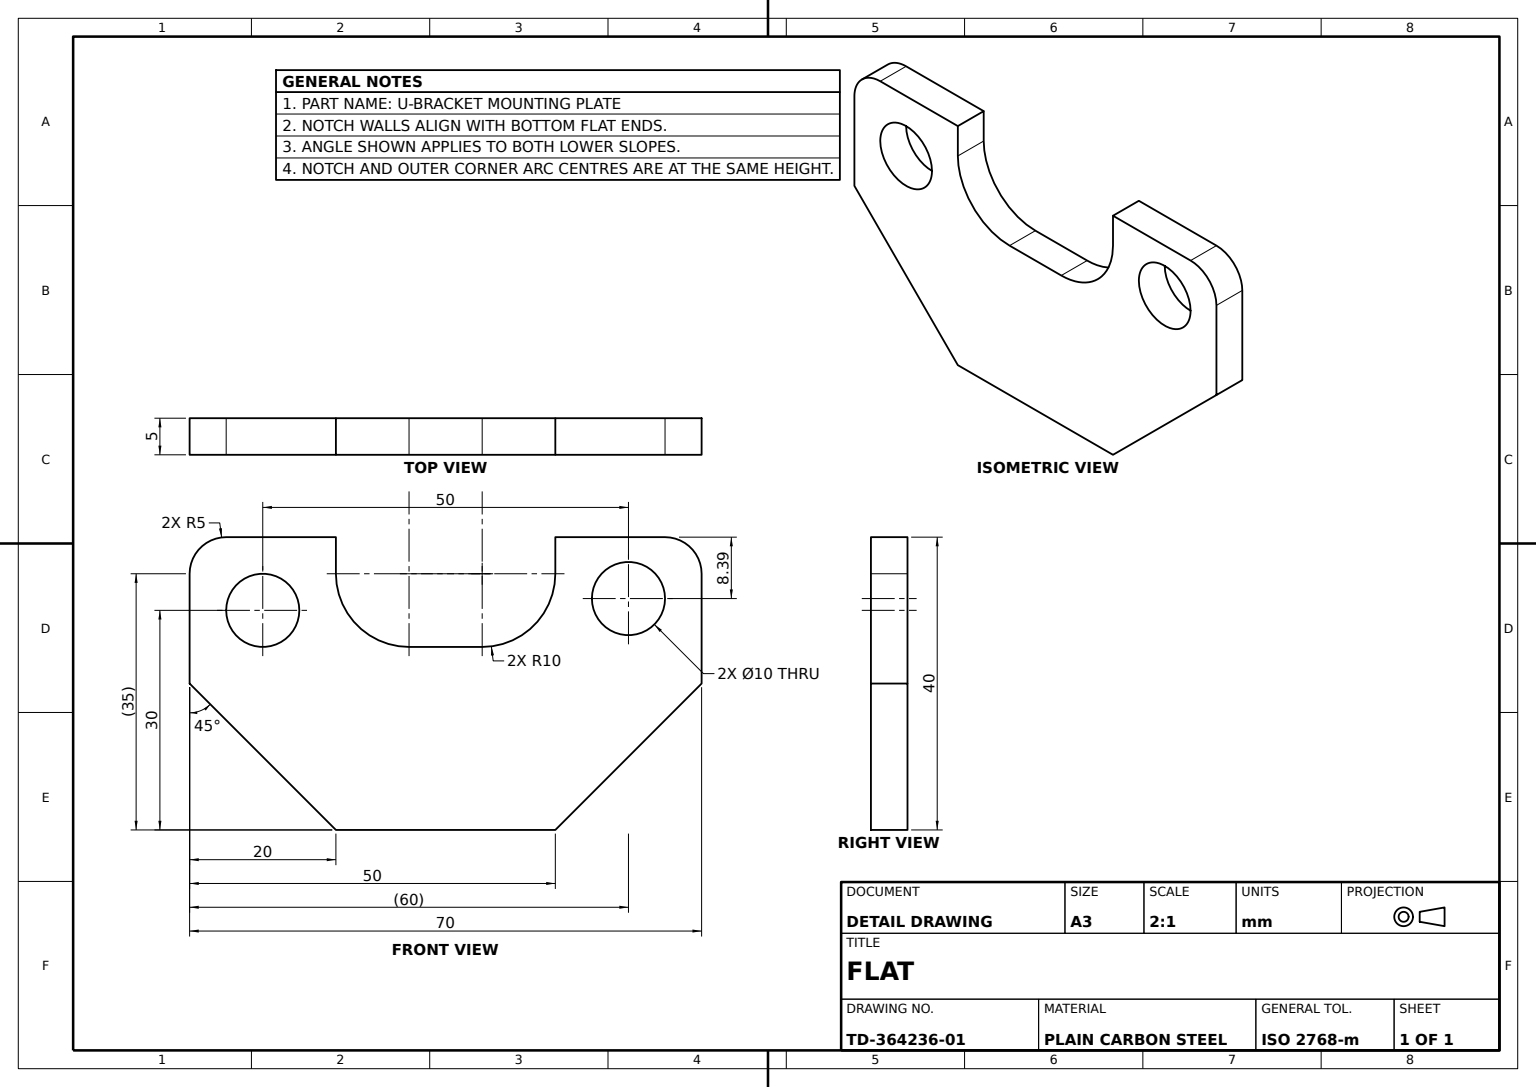
SolidWorks part; units mm, degrees
material "Plain Carbon Steel"
ref_plane "Front Plane" through (0, 0, 0) normal (0, 0, 1) x (1, 0, 0)
ref_plane "Top Plane" through (0, 0, 0) normal (0, 1, 0) x (1, 0, 0)
ref_plane "Right Plane" through (0, 0, 0) normal (1, 0, 0) x (0, 0, -1)
sketch "Bracket Profile Sketch" plane through (0, 0, 0) normal (0, 0, 1) x (1, 0, 0)
  line L0 (0, 0) -> (30, 0)
  line L1 (0, 40) -> (0, 35)
  line L2 (10, 25) -> (20, 25)
  line L3 (30, 35) -> (30, 40)
  line L4 (0, 40) -> (-20, 40)
  line L5 (-20, 40) -> (-20, 20)
  line L6 (30, 40) -> (50, 40)
  line L7 (50, 40) -> (50, 20)
  line L8 (0, 0) -> (-20, 20)
  line L9 (30, 0) -> (50, 20)
  arc A0 (0, 35) -> (10, 25) centre (10, 35) ccw
  arc A1 (20, 25) -> (30, 35) centre (20, 35) ccw
  dimension "D7" = 50
  dimension "D9" = 20
  dimension "D1" = 30
  dimension "D2" = 20
  dimension "D3" = 20
  dimension "D4" = 20
  dimension "D5" = 20
  dimension "D6" = 20
  dimension "D8" = 35
  dimension "D10" = 20
extrude "Bracket Plate" add sketch "Bracket Profile Sketch" along normal blind 5
sketch "Mounting Hole A Sketch" plane through (0, 0, 5) normal (0, 0, 1) x (1, 0, 0)
  line L0 (0, 0) -> (30, 0) construction
  line L1 (50, 20) -> (50, 40) construction
  circle A0 centre (-10, 30) radius 5
  dimension "D1" = 10
  dimension "D2" = 30
  dimension "D3" = 60
extrude "Mounting Hole A Ø10" cut sketch "Mounting Hole A Sketch" against normal blind 5
sketch "Mounting Hole B Sketch" plane through (0, 0, 5) normal (0, 0, 1) x (1, 0, 0)
  line L0 (50, 20) -> (50, 40) construction
  line L1 (50, 40) -> (30, 40) construction
  circle A0 centre (40, 31.6095) radius 5
  dimension "D1" = 10
  dimension "D2" = 10
  dimension "D3" = 8.3905
extrude "Mounting Hole B Ø10" cut sketch "Mounting Hole B Sketch" against normal blind 5
fillet "Corner Fillets R5" radius 5 2 edges at (50, 40, 2.5) (-20, 40, 2.5)
